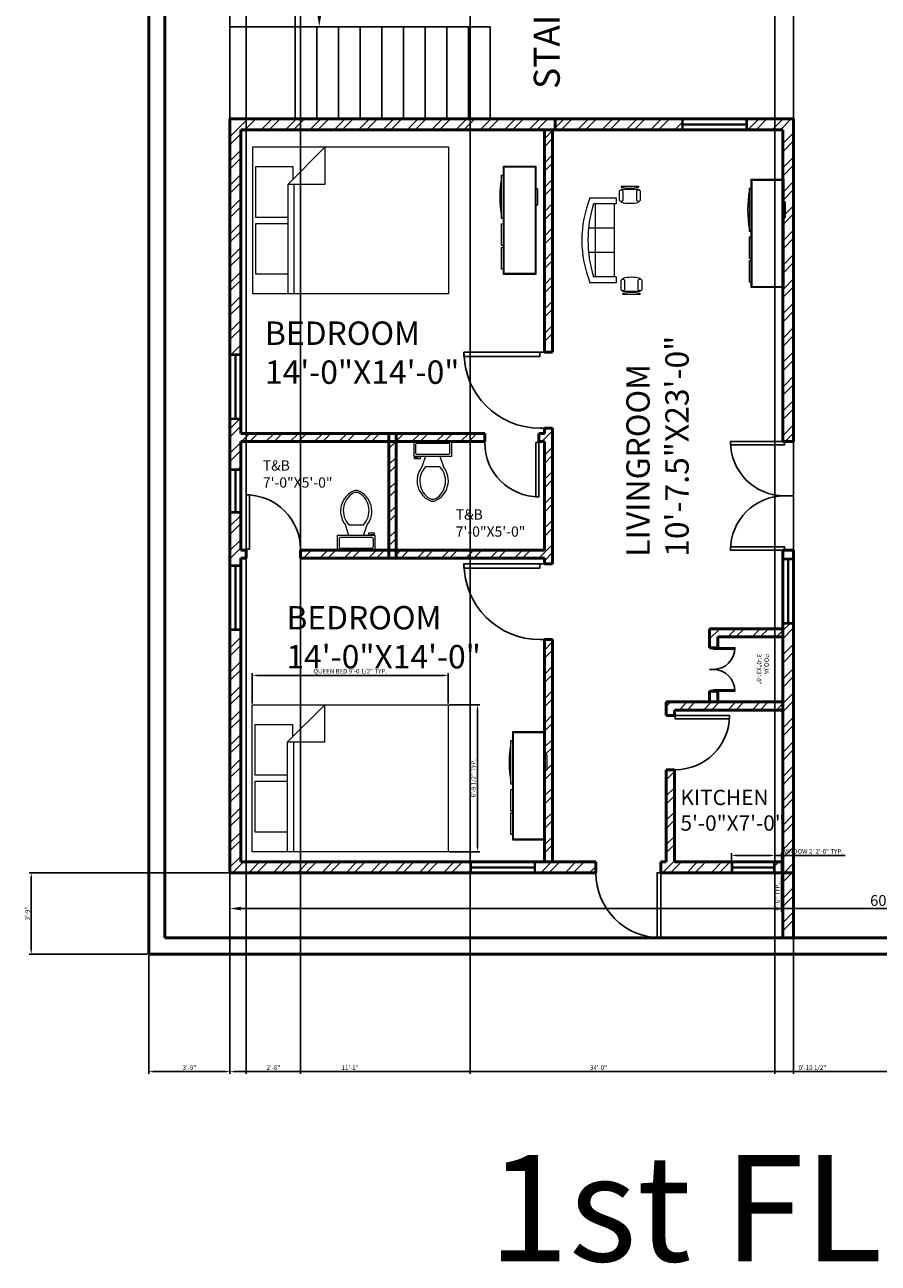
# Model space of a CAD drawing. Units: inches. Extents: x -12550 to 6516, y 1273 to 18700.
# Tile 2 of 19: x 1904 to 2377, y 1273 to 1958. Entities that reach past the tile are written whole.
import ezdxf

# ---------------------------------------------------------------- set-up
doc = ezdxf.new("R2010")
doc.units = ezdxf.units.IN
for name, color, linetype, lineweight in [('A-ANNO-DIMS', 2, 'Continuous', 18), ('A-ANNO-TEXT', 7, 'Continuous', 25), ('A-AREA-IDEN', 1, 'Continuous', 18), ('A-DOOR', 5, 'Continuous', 25), ('A-FLOR-STRS', 6, 'Continuous', 25), ('A-FURN', 8, 'Continuous', 18), ('A-GLAZ', 3, 'Continuous', 25), ('A-WALL', 7, 'Continuous', 50), ('A-WALL-PATT', 8, 'Continuous', 13)]:
    doc.layers.add(name, color=color, linetype=linetype, lineweight=lineweight)
doc.styles.get("Standard").update_dxf_attribs({"font": 'arial.ttf'})
doc.dimstyles.new('ISO-25', dxfattribs={"dimtxt": 2.5, "dimasz": 2.5, "dimexe": 1.25, "dimexo": 0.625, "dimtad": 1, "dimlunit": 4, "dimtxsty": 'Standard', "dimcen": 2.5, "dimadec": 0, "dimazin": 0, "dimtfac": 1, "dimtmove": 0, "dimatfit": 3, "dimfxl": 1, "dimarcsym": 0})

# ---------------------------------------------------------------- blocks, each defined once
blk = doc.blocks.new('*U2')
for p, q in [((0, 0), (0, -5)), ((30, 0), (30, -5))]:
    blk.add_line(p, q)
blk.add_lwpolyline([(0, 0), (0, 30), (1.75, 30), (1.75, 0)], close=True)
blk.add_arc((0, 0), 30, 0, 90)
blk = doc.blocks.new('Bed - Queen')
for p, q in [((0, -80.00003), (0, 0)), ((0, 0), (59.99999, 0)), ((59.99999, 0), (59.99999, -80.00003)), ((7.99999, -1.2), (28.79998, -1.2)), ((7.99999, -14.4), (7.99999, -1.2)), ((28.79998, -1.2), (28.79998, -14.4)), ((31.19999, -1.2), (51.99999, -1.2)), ((31.19999, -14.4), (31.19999, -1.2)), ((51.99999, -1.2), (51.99999, -16.4)), ((0, -14.4), (44.8, -14.4)), ((59.99999, -29.6), (44.8, -14.4)), ((44.8, -14.4), (44.8, -29.6)), ((44.8, -16.8), (0, -16.8)), ((51.99999, -16.4), (46.79936, -16.4)), ((44.8, -29.6), (59.99999, -29.6)), ((59.99999, -80.00003), (0, -80.00003))]:
    blk.add_line(p, q)
blk = doc.blocks.new('Toilet - top')
for p, q in [((9.5, -6), (9.5, -2)), ((-10, -8.5), (-8, -8.5)), ((-10, -9.5), (-10, -8.5)), ((-7, -9.5), (-10, -9.5)), ((-8, -8.5), (-8, -8)), ((-7, -8), (-7, -9.5)), ((-4, -8), (-6, -14)), ((4, -8), (6, -14)), ((4, -14), (-4, -14))]:
    blk.add_line(p, q)
blk.add_lwpolyline([(10.5, -8), (10.5, 0), (-10.5, 0), (-10.5, -8)], close=True)
for points in [[(-9.5, -2), (-9.5, -6)], [(8.5, -1), (-8.5, -1)], [(-8.5, -7), (8.5, -7)]]:
    blk.add_lwpolyline(points)
for centre, radius, start, end in [((-8.62, -1.88), 0.884, 81.8699, 188.1301), ((-8.62, -6.12), 0.884, 171.8699, 278.1301), ((8.62, -1.88), 0.884, 351.8699, 98.1301), ((8.62, -6.12), 0.884, 261.8699, 8.1301), ((3.52, -21.58), 12.17, 141.46911, 247.97143), ((4.2, -21.82), 11.33, 136.36773, 238.94682), ((-3.52, -21.58), 12.17, 292.02843, 38.53071), ((-4.2, -21.82), 11.33, 301.05301, 43.63209), ((0, -27.88), 4, 245.73182, 294.26817), ((0, -29), 4, 254.86053, 285.13947)]:
    blk.add_arc(centre, radius, start, end)
blk = doc.blocks.new('Entertainment Center')
for p, q in [((-4, 0), (-5, -1)), ((4, 0), (-4, 0)), ((5, -1), (4, 0)), ((-17, -19), (-17, -1)), ((-17, -1), (43, -1)), ((-16.5, -18.5), (-16.5, -1.5)), ((-16.5, -1.5), (42.5, -1.5)), ((42.5, -1.5), (42.5, -18.5)), ((43, -1), (43, -19)), ((43, -19), (-17, -19)), ((42.5, -18.5), (-16.5, -18.5)), ((-12, -20), (-12, -19)), ((12, -20), (-12, -20)), ((12, -19), (12, -20)), ((15, -20), (15, -19)), ((27, -20), (15, -20)), ((27, -19), (27, -20)), ((28, -20), (28, -19)), ((40, -20), (28, -20)), ((40, -19), (40, -20))]:
    blk.add_line(p, q)
blk.add_arc((0, 40), 61, 259.6111, 280.3889)
blk = doc.blocks.new('Sofa - Roundback 7 ft.')
for p, q in [((-36.000027, -34), (-36.000027, -11.4696)), ((-12.00002, -32.4421), (-12.00003, -6.5971)), ((11.99997, -32.4421), (11.99998, -6.5971)), ((35.99998, -34), (35.99998, -11.4696)), ((-35.999844, -13.3819), (35.9998, -13.3819)), ((-36.000027, -32.4421), (35.99998, -32.4421))]:
    blk.add_line(p, q)
for points in [[(-36.000027, -34), (-42.000027, -34), (-42.000027, -8)], [(41.99998, -8), (41.99998, -34), (35.99998, -34)]]:
    blk.add_lwpolyline(points)
for centre, radius, start, end in [((0, -114.25), 114.25, 68.43141, 111.5686), ((-0.00001, -127.1968), 121.1968, 72.72033, 107.2797)]:
    blk.add_arc(centre, radius, start, end)
blk = doc.blocks.new('Chair - Desk')
for p, q in [((-8.5, 0), (-8.5, -1)), ((-8.5, 0), (8.5, 0)), ((8.5, 0), (8.5, -1)), ((-10.5, -5), (-10.5, -14)), ((-8.5, -3), (-8.5, -4)), ((-8.5, -3), (8.5, -3)), ((-6.5, -14), (-6.5, -5)), ((-2, -3), (-2, -1.9355)), ((2, -1.9576), (2, -3)), ((6.5, -5), (6.5, -14)), ((8.5, -3), (8.5, -4)), ((10.5, -14), (10.5, -5)), ((-8.5, -15), (-8.5, -16)), ((8.5, -15), (8.5, -16))]:
    blk.add_line(p, q)
for centre, radius, start, end in [((-8.5, -6.5), 2.5, 36.8699, 143.1301), ((0, 34.625), 36.625, 256.5803, 283.4197), ((8.5, -6.5), 2.5, 36.8699, 143.1301), ((-8.5, -12.5), 2.5, 216.8699, 323.1301), ((0, 19.625), 36.625, 256.5803, 283.4197), ((8.5, -12.5), 2.5, 216.8699, 323.1301)]:
    blk.add_arc(centre, radius, start, end)
blk = doc.blocks.new('*D13')
at = {"layer": 'A-ANNO-DIMS', "color": 0, "lineweight": -2, "transparency": 16777216}
for p, q in [((2054.31, 2008.25), (2068.36, 2008.25)), ((2067.11, 2002.25), (2067.11, 1963.25)), ((2054.31, 1957.25), (2068.36, 1957.25))]:
    blk.add_line(p, q, dxfattribs=at)
at = {"layer": 'A-ANNO-DIMS', "color": 0, "transparency": 16777216}
for points in [[(2066.11, 2002.25), (2068.11, 2002.25), (2067.11, 2008.25)], [(2066.11, 1963.25), (2068.11, 1963.25), (2067.11, 1957.25)]]:
    blk.add_solid(points, dxfattribs=at)
at = {"layer": 'Defpoints', "color": 0, "transparency": 16777216}
for p in [(2053.69, 2008.25), (2053.69, 1957.25), (2067.11, 1957.25)]:
    blk.add_point(p, dxfattribs=at)
at = {"layer": 'A-ANNO-DIMS', "color": 0, "transparency": 16777216, "insert": (2063.42, 1982.75), "char_height": 6, "attachment_point": 5, "rotation": 90}
blk.add_mtext('4\'-3"', dxfattribs=at)
blk = doc.blocks.new('*D17')
at = {"layer": 'A-ANNO-DIMS', "color": 0, "lineweight": -2, "transparency": 16777216}
for p, q in [((2017.69, 1488.62), (2017.69, 1468.21)), ((2737.69, 1488.62), (2737.69, 1468.21)), ((2731.69, 1469.46), (2023.69, 1469.46))]:
    blk.add_line(p, q, dxfattribs=at)
at = {"layer": 'A-ANNO-DIMS', "color": 0, "transparency": 16777216}
for points in [[(2023.69, 1470.46), (2023.69, 1468.46), (2017.69, 1469.46)], [(2731.69, 1470.46), (2731.69, 1468.46), (2737.69, 1469.46)]]:
    blk.add_solid(points, dxfattribs=at)
at = {"layer": 'Defpoints', "color": 0, "transparency": 16777216}
for p in [(2017.69, 1489.25), (2737.69, 1489.25), (2017.69, 1469.46)]:
    blk.add_point(p, dxfattribs=at)
at = {"layer": 'A-ANNO-DIMS', "color": 0, "transparency": 16777216, "insert": (2377.69, 1473.15), "char_height": 6, "attachment_point": 5}
blk.add_mtext("60'", dxfattribs=at)
blk = doc.blocks.new('WIN-3FT')
for p, q in [((0, 0), (0, 6)), ((0, 6), (36.02, 6)), ((36.02, 0), (0, 0)), ((0.5, 0), (0.5, 6)), ((35.52, 3.2), (0.5, 3.2)), ((35.52, 2.8), (0.5, 2.8)), ((35.52, 6), (35.52, 0)), ((36.02, 6), (36.02, 0))]:
    blk.add_line(p, q)
blk = doc.blocks.new('WIN-2FT')
for p, q in [((0, 0), (0, 24.02)), ((0, 24.02), (6, 24.02)), ((0, 23.52), (6, 23.52)), ((2.8, 0.5), (2.8, 23.52)), ((3.2, 0.5), (3.2, 23.52)), ((6, 24.02), (6, 0)), ((6, 0.5), (0, 0.5)), ((6, 0), (0, 0))]:
    blk.add_line(p, q)
blk = doc.blocks.new('*D65')
at = {"layer": 'A-ANNO-DIMS', "color": 0, "lineweight": -2, "transparency": 16777216}
for p, q in [((2295.28, 1495.87), (2295.28, 1500.1)), ((2297.78, 1498.85), (2316.79, 1498.85)), ((2319.29, 1495.87), (2319.29, 1500.1)), ((2319.29, 1498.85), (2358.26, 1498.85))]:
    blk.add_line(p, q, dxfattribs=at)
at = {"layer": 'A-ANNO-DIMS', "color": 0, "transparency": 16777216}
for points in [[(2297.78, 1499.27), (2297.78, 1498.43), (2295.28, 1498.85)], [(2316.79, 1499.27), (2316.79, 1498.43), (2319.29, 1498.85)]]:
    blk.add_solid(points, dxfattribs=at)
at = {"layer": 'Defpoints', "color": 0, "transparency": 16777216}
for p in [(2295.28, 1495.25), (2319.29, 1498.85), (2319.29, 1495.25)]:
    blk.add_point(p, dxfattribs=at)
at = {"layer": 'A-ANNO-DIMS', "color": 0, "transparency": 16777216, "insert": (2340.03, 1500.77), "char_height": 2.5, "attachment_point": 5}
blk.add_mtext('WINDOW 2\' 2\'-0" TYP.', dxfattribs=at)
blk = doc.blocks.new('*D66')
at = {"layer": 'A-ANNO-DIMS', "color": 0, "lineweight": -2, "transparency": 16777216}
for p, q in [((2319.92, 1495.25), (2324.15, 1495.25)), ((2322.9, 1497.75), (2322.9, 1500.25)), ((2322.9, 1495.25), (2322.9, 1489.25)), ((2319.92, 1489.25), (2324.15, 1489.25)), ((2322.9, 1486.75), (2322.9, 1467.76))]:
    blk.add_line(p, q, dxfattribs=at)
at = {"layer": 'A-ANNO-DIMS', "color": 0, "transparency": 16777216}
for points in [[(2322.48, 1497.75), (2323.31, 1497.75), (2322.9, 1495.25)], [(2322.48, 1486.75), (2323.31, 1486.75), (2322.9, 1489.25)]]:
    blk.add_solid(points, dxfattribs=at)
at = {"layer": 'Defpoints', "color": 0, "transparency": 16777216}
for p in [(2319.29, 1495.25), (2319.29, 1489.25), (2322.9, 1489.25)]:
    blk.add_point(p, dxfattribs=at)
at = {"layer": 'A-ANNO-DIMS', "color": 0, "transparency": 16777216, "insert": (2321, 1476), "char_height": 2.5, "attachment_point": 5, "rotation": 90}
blk.add_mtext('0\'-6" TYP.', dxfattribs=at)
blk = doc.blocks.new('*D69')
at = {"layer": 'A-ANNO-DIMS', "color": 0, "lineweight": -2, "transparency": 16777216}
for p, q in [((2030.04, 1582.83), (2030.04, 1599.71)), ((2135.92, 1598.46), (2032.54, 1598.46)), ((2138.42, 1582.83), (2138.42, 1599.71))]:
    blk.add_line(p, q, dxfattribs=at)
at = {"layer": 'A-ANNO-DIMS', "color": 0, "transparency": 16777216}
for points in [[(2032.54, 1598.88), (2032.54, 1598.05), (2030.04, 1598.46)], [(2135.92, 1598.88), (2135.92, 1598.05), (2138.42, 1598.46)]]:
    blk.add_solid(points, dxfattribs=at)
at = {"layer": 'Defpoints', "color": 0, "transparency": 16777216}
for p in [(2030.04, 1598.46), (2030.04, 1582.2), (2138.42, 1582.2)]:
    blk.add_point(p, dxfattribs=at)
at = {"layer": 'A-ANNO-DIMS', "color": 0, "transparency": 16777216, "insert": (2084.23, 1600.46), "char_height": 2.5, "attachment_point": 5}
blk.add_mtext('QUEEN BED 9\'-0 1/2" TYP.', dxfattribs=at)
blk = doc.blocks.new('*D70')
at = {"layer": 'A-ANNO-DIMS', "color": 0, "lineweight": -2, "transparency": 16777216}
for p, q in [((2139.05, 1582.2), (2155.93, 1582.2)), ((2154.68, 1503.41), (2154.68, 1579.7)), ((2139.05, 1500.91), (2155.93, 1500.91))]:
    blk.add_line(p, q, dxfattribs=at)
at = {"layer": 'A-ANNO-DIMS', "color": 0, "transparency": 16777216}
for points in [[(2154.27, 1579.7), (2155.1, 1579.7), (2154.68, 1582.2)], [(2154.27, 1503.41), (2155.1, 1503.41), (2154.68, 1500.91)]]:
    blk.add_solid(points, dxfattribs=at)
at = {"layer": 'Defpoints', "color": 0, "transparency": 16777216}
for p in [(2138.42, 1582.2), (2154.68, 1582.2), (2138.42, 1500.91)]:
    blk.add_point(p, dxfattribs=at)
at = {"layer": 'A-ANNO-DIMS', "color": 0, "transparency": 16777216, "insert": (2152.76, 1541.56), "char_height": 2.5, "attachment_point": 5, "rotation": 90}
blk.add_mtext('6\'-9 1/2" TYP.', dxfattribs=at)
blk = doc.blocks.new('*D96')
at = {"layer": 'A-ANNO-DIMS', "color": 0, "lineweight": -2, "transparency": 16777216}
for p, q in [((2017.69, 1488.62), (2017.69, 1378)), ((1972.69, 1443.62), (1972.69, 1378)), ((1975.19, 1379.25), (2015.19, 1379.25))]:
    blk.add_line(p, q, dxfattribs=at)
at = {"layer": 'A-ANNO-DIMS', "color": 0, "transparency": 16777216}
for points in [[(1975.19, 1379.66), (1975.19, 1378.83), (1972.69, 1379.25)], [(2015.19, 1379.66), (2015.19, 1378.83), (2017.69, 1379.25)]]:
    blk.add_solid(points, dxfattribs=at)
at = {"layer": 'Defpoints', "color": 0, "transparency": 16777216}
for p in [(2017.69, 1489.25), (1972.69, 1444.25), (2017.69, 1379.25)]:
    blk.add_point(p, dxfattribs=at)
at = {"layer": 'A-ANNO-DIMS', "color": 0, "transparency": 16777216, "insert": (1995.19, 1381.15), "char_height": 2.5, "attachment_point": 5}
blk.add_mtext('3\'-9"', dxfattribs=at)
blk = doc.blocks.new('*D97')
at = {"layer": 'A-ANNO-DIMS', "color": 0, "lineweight": -2, "transparency": 16777216}
for p, q in [((2017.69, 1488.62), (2017.69, 1378)), ((2425.69, 1488.62), (2425.69, 1378)), ((2020.19, 1379.25), (2423.19, 1379.25))]:
    blk.add_line(p, q, dxfattribs=at)
at = {"layer": 'A-ANNO-DIMS', "color": 0, "transparency": 16777216}
for points in [[(2020.19, 1379.66), (2020.19, 1378.83), (2017.69, 1379.25)], [(2423.19, 1379.66), (2423.19, 1378.83), (2425.69, 1379.25)]]:
    blk.add_solid(points, dxfattribs=at)
at = {"layer": 'Defpoints', "color": 0, "transparency": 16777216}
for p in [(2017.69, 1489.25), (2425.69, 1489.25), (2425.69, 1379.25)]:
    blk.add_point(p, dxfattribs=at)
at = {"layer": 'A-ANNO-DIMS', "color": 0, "transparency": 16777216, "insert": (2221.69, 1381.15), "char_height": 2.5, "attachment_point": 5}
blk.add_mtext('34\'-0"', dxfattribs=at)
blk = doc.blocks.new('*D101')
at = {"layer": 'A-ANNO-DIMS', "color": 0, "lineweight": -2, "transparency": 16777216}
for p, q in [((2017.06, 1489.25), (1906.44, 1489.25)), ((1907.69, 1446.75), (1907.69, 1486.75)), ((1972.06, 1444.25), (1906.44, 1444.25))]:
    blk.add_line(p, q, dxfattribs=at)
at = {"layer": 'A-ANNO-DIMS', "color": 0, "transparency": 16777216}
for points in [[(1907.27, 1486.75), (1908.11, 1486.75), (1907.69, 1489.25)], [(1907.27, 1446.75), (1908.11, 1446.75), (1907.69, 1444.25)]]:
    blk.add_solid(points, dxfattribs=at)
at = {"layer": 'Defpoints', "color": 0, "transparency": 16777216}
for p in [(1907.69, 1489.25), (2017.69, 1489.25), (1972.69, 1444.25)]:
    blk.add_point(p, dxfattribs=at)
at = {"layer": 'A-ANNO-DIMS', "color": 0, "transparency": 16777216, "insert": (1905.79, 1466.75), "char_height": 2.5, "attachment_point": 5, "rotation": 90}
blk.add_mtext('3\'-9"', dxfattribs=at)
blk = doc.blocks.new('*D136')
at = {"layer": 'A-ANNO-DIMS', "color": 0, "lineweight": -2, "transparency": 16777216}
for p, q in [((2017.69, 2055.62), (2017.69, 1378)), ((2150.64, 2055.62), (2150.64, 1378)), ((2020.19, 1379.25), (2148.14, 1379.25))]:
    blk.add_line(p, q, dxfattribs=at)
at = {"layer": 'A-ANNO-DIMS', "color": 0, "transparency": 16777216}
for points in [[(2020.19, 1379.66), (2020.19, 1378.83), (2017.69, 1379.25)], [(2148.14, 1379.66), (2148.14, 1378.83), (2150.64, 1379.25)]]:
    blk.add_solid(points, dxfattribs=at)
at = {"layer": 'Defpoints', "color": 0, "transparency": 16777216}
for p in [(2017.69, 2056.25), (2150.64, 2056.25), (2150.64, 1379.25)]:
    blk.add_point(p, dxfattribs=at)
at = {"layer": 'A-ANNO-DIMS', "color": 0, "transparency": 16777216, "insert": (2084.16, 1381.13), "char_height": 2.5, "attachment_point": 5}
blk.add_mtext('11\'-1"', dxfattribs=at)
blk = doc.blocks.new('*D137')
at = {"layer": 'A-ANNO-DIMS', "color": 0, "lineweight": -2, "transparency": 16777216}
for p, q in [((2319.29, 2055.62), (2319.29, 1378)), ((2329.69, 2055.62), (2329.69, 1378)), ((2321.79, 1379.25), (2327.19, 1379.25)), ((2329.69, 1379.25), (2347.85, 1379.25))]:
    blk.add_line(p, q, dxfattribs=at)
at = {"layer": 'A-ANNO-DIMS', "color": 0, "transparency": 16777216}
for points in [[(2321.79, 1379.66), (2321.79, 1378.83), (2319.29, 1379.25)], [(2327.19, 1379.66), (2327.19, 1378.83), (2329.69, 1379.25)]]:
    blk.add_solid(points, dxfattribs=at)
at = {"layer": 'Defpoints', "color": 0, "transparency": 16777216}
for p in [(2319.29, 2056.25), (2329.69, 2056.25), (2329.69, 1379.25)]:
    blk.add_point(p, dxfattribs=at)
at = {"layer": 'A-ANNO-DIMS', "color": 0, "transparency": 16777216, "insert": (2340.02, 1381.16), "char_height": 2.5, "attachment_point": 5}
blk.add_mtext('0\'-10 1/2"', dxfattribs=at)
blk = doc.blocks.new('*D142')
at = {"layer": 'A-ANNO-DIMS', "color": 0, "lineweight": -2, "transparency": 16777216}
for p, q in [((2026.69, 2234.12), (2026.69, 1378)), ((2056.69, 2234.12), (2056.69, 1378)), ((2029.19, 1379.25), (2054.19, 1379.25))]:
    blk.add_line(p, q, dxfattribs=at)
at = {"layer": 'A-ANNO-DIMS', "color": 0, "transparency": 16777216}
for points in [[(2029.19, 1379.66), (2029.19, 1378.83), (2026.69, 1379.25)], [(2054.19, 1379.66), (2054.19, 1378.83), (2056.69, 1379.25)]]:
    blk.add_solid(points, dxfattribs=at)
at = {"layer": 'Defpoints', "color": 0, "transparency": 16777216}
for p in [(2026.69, 2234.75), (2056.69, 2234.75), (2056.69, 1379.25)]:
    blk.add_point(p, dxfattribs=at)
at = {"layer": 'A-ANNO-DIMS', "color": 0, "transparency": 16777216, "insert": (2041.69, 1381.15), "char_height": 2.5, "attachment_point": 5}
blk.add_mtext('2\'-6"', dxfattribs=at)

msp = doc.modelspace()

# ---------------------------------------------------------------- hatches: boundary and pattern name
at = {"layer": 'A-WALL-PATT'}
h = msp.add_hatch(dxfattribs=at)
h.set_pattern_fill('ANSI32', color=256)
h.paths.add_polyline_path([(2023.689, 1900.247), (2197.689, 1900.247), (2197.689, 1906.247), (2017.689, 1906.247), (2017.689, 1776.138), (2023.689, 1776.138)])
h = msp.add_hatch(dxfattribs=at)
h.set_pattern_fill('ANSI32', color=256)
h.paths.add_polyline_path([(2267.94, 1906.247), (2197.689, 1906.247), (2197.689, 1900.247), (2267.94, 1900.247)])
h = msp.add_hatch(dxfattribs=at)
h.set_pattern_fill('ANSI32', color=256)
h.paths.add_polyline_path([(2329.689, 1906.247), (2303.958, 1906.247), (2303.958, 1900.247), (2323.689, 1900.247), (2323.689, 1872.972), (2324.189, 1872.972), (2324.189, 1860.972), (2325.189, 1859.972), (2325.189, 1851.972), (2324.189, 1850.972), (2324.189, 1812.972), (2323.689, 1727.747), (2324.689, 1727.747), (2329.689, 1727.747)])
h = msp.add_hatch(dxfattribs=at)
h.set_pattern_fill('ANSI32', color=256)
h.paths.add_polyline_path([(2196.189, 1900.247), (2191.689, 1900.247), (2191.689, 1777.247), (2196.189, 1777.247)], flags=17)
h = msp.add_hatch(dxfattribs=at)
h.set_pattern_fill('ANSI32', color=256)
h.paths.add_polyline_path([(2105.689, 1732.247), (2023.689, 1732.247), (2023.689, 1740.121), (2017.689, 1740.121), (2017.689, 1712.466), (2023.689, 1712.466), (2023.689, 1727.747), (2105.689, 1727.747)])
h = msp.add_hatch(dxfattribs=at)
h.set_pattern_fill('ANSI32', color=256)
h.paths.add_polyline_path([(2196.189, 1735.247), (2191.689, 1735.247), (2191.689, 1732.247), (2188.689, 1732.247), (2188.689, 1727.747), (2191.689, 1727.747), (2191.689, 1667.747), (2109.689, 1667.747), (2109.689, 1663.247), (2191.689, 1663.247), (2191.689, 1660.247), (2196.189, 1660.247)])
h = msp.add_hatch(dxfattribs=at)
h.set_pattern_fill('ANSI32', color=256)
h.paths.add_polyline_path([(2109.689, 1727.747), (2105.689, 1727.747), (2105.689, 1667.747), (2109.689, 1667.747)])
h = msp.add_hatch(dxfattribs=at)
h.set_pattern_fill('ANSI32', color=256)
h.paths.add_polyline_path([(2158.689, 1732.247), (2109.689, 1732.247), (2109.689, 1727.747), (2158.689, 1727.747)], flags=17)
h = msp.add_hatch(dxfattribs=at)
h.set_pattern_fill('ANSI32', color=256)
h.paths.add_polyline_path([(2023.689, 1688.449), (2017.689, 1688.449), (2017.689, 1659.453), (2023.689, 1659.453), (2023.689, 1663.247), (2026.689, 1663.247), (2026.689, 1667.747), (2023.689, 1667.747)])
h = msp.add_hatch(dxfattribs=at)
h.set_pattern_fill('ANSI32', color=256)
h.paths.add_polyline_path([(2105.689, 1667.747), (2056.689, 1667.747), (2056.689, 1663.247), (2105.689, 1663.247)])
h = msp.add_hatch(dxfattribs=at)
h.set_pattern_fill('ANSI32', color=256)
h.paths.add_polyline_path([(2323.689, 1624.247), (2283.189, 1624.247), (2283.189, 1613.747), (2285.189, 1613.747), (2287.689, 1613.747), (2287.689, 1619.747), (2323.689, 1619.747)])
h = msp.add_hatch(dxfattribs=at)
h.set_pattern_fill('ANSI32', color=256)
h.paths.add_polyline_path([(2329.689, 1627.032), (2323.689, 1627.032), (2323.689, 1495.247), (2319.294, 1495.247), (2319.294, 1489.247), (2329.689, 1489.247)])
h = msp.add_hatch(dxfattribs=at)
h.set_pattern_fill('ANSI32', color=256)
h.paths.add_polyline_path([(2023.689, 1623.435), (2017.689, 1623.435), (2017.689, 1489.247), (2150.64, 1489.247), (2150.64, 1495.247), (2023.689, 1495.247)])
h = msp.add_hatch(dxfattribs=at)
h.set_pattern_fill('ANSI32', color=256)
h.paths.add_polyline_path([(2196.189, 1618.247), (2191.689, 1618.247), (2191.689, 1567.365), (2192.189, 1567.365), (2192.189, 1555.365), (2193.189, 1554.365), (2193.189, 1546.365), (2192.189, 1545.365), (2192.189, 1507.365), (2191.689, 1495.247), (2196.189, 1495.247)])
h = msp.add_hatch(dxfattribs=at)
h.set_pattern_fill('ANSI32', color=256)
h.paths.add_polyline_path([(2323.689, 1583.747), (2259.189, 1583.747), (2259.189, 1576.247), (2263.689, 1576.247), (2263.689, 1579.247), (2323.689, 1579.247)])
h = msp.add_hatch(dxfattribs=at)
h.set_pattern_fill('ANSI32', color=256)
h.paths.add_polyline_path([(2295.277, 1495.247), (2263.689, 1495.247), (2263.689, 1546.247), (2259.189, 1546.247), (2259.189, 1495.247), (2256.189, 1495.247), (2256.189, 1489.247), (2295.277, 1489.247)])
h = msp.add_hatch(dxfattribs=at)
h.set_pattern_fill('ANSI32', color=256)
h.paths.add_polyline_path([(2220.189, 1495.247), (2186.657, 1495.247), (2186.657, 1489.247), (2220.189, 1489.247)])
h = msp.add_hatch(dxfattribs=at)
h.set_pattern_fill('ANSI32', color=256)
h.paths.add_polyline_path([(2329.689, 1489.247), (2323.689, 1489.247), (2323.689, 1453.247), (2329.689, 1453.247)])

# ---------------------------------------------------------------- linework, layer by layer
at = {"layer": 'A-FLOR-STRS'}
for p, q in [((2017.689, 2056.247), (2017.689, 1906.247)), ((2053.689, 2056.247), (2053.689, 1906.247)), ((2017.689, 1957.247), (2161.689, 1957.247)), ((2065.689, 1957.247), (2065.689, 1906.247)), ((2077.689, 1957.247), (2077.689, 1906.247)), ((2089.689, 1957.247), (2089.689, 1906.247)), ((2101.689, 1957.247), (2101.689, 1906.247)), ((2113.689, 1957.247), (2113.689, 1906.247)), ((2125.689, 1957.247), (2125.689, 1906.247)), ((2137.689, 1957.247), (2137.689, 1906.247)), ((2149.689, 1957.247), (2149.689, 1906.247)), ((2161.689, 1957.247), (2161.689, 1906.247)), ((2017.689, 1906.247), (2197.689, 1906.247))]:
    msp.add_line(p, q, dxfattribs=at)
at = {"layer": 'A-WALL'}
for p, q in [((1972.689, 1444.247), (1972.689, 2518.247)), ((1981.689, 1453.247), (1981.689, 2509.247)), ((2017.689, 1489.247), (2017.689, 1906.247)), ((2329.689, 1906.247), (2017.689, 1906.247)), ((2197.689, 1900.247), (2197.689, 1906.247)), ((2329.689, 1727.747), (2329.689, 1906.247)), ((2023.689, 1732.247), (2023.689, 1900.247)), ((2323.689, 1900.247), (2023.689, 1900.247)), ((2191.689, 1777.247), (2191.689, 1900.247)), ((2196.189, 1777.247), (2196.189, 1900.247)), ((2323.689, 1727.747), (2323.689, 1900.247)), ((2196.189, 1777.247), (2191.689, 1777.247)), ((2191.689, 1732.247), (2191.689, 1735.247)), ((2191.689, 1735.247), (2196.189, 1735.247)), ((2191.689, 1732.247), (2191.689, 1735.247)), ((2196.189, 1660.247), (2196.189, 1735.247)), ((2158.689, 1732.247), (2023.689, 1732.247)), ((2158.689, 1727.747), (2023.689, 1727.747)), ((2023.689, 1667.747), (2023.689, 1727.747)), ((2105.689, 1663.247), (2105.689, 1732.247)), ((2109.689, 1663.247), (2109.689, 1732.247)), ((2158.689, 1727.747), (2158.689, 1732.247)), ((2191.689, 1732.247), (2188.689, 1732.247)), ((2191.689, 1732.247), (2188.689, 1732.247)), ((2188.689, 1732.247), (2188.689, 1727.747)), ((2191.689, 1727.747), (2188.689, 1727.747)), ((2191.689, 1667.747), (2191.689, 1727.747)), ((2329.689, 1727.747), (2323.689, 1727.747)), ((2026.689, 1667.747), (2023.689, 1667.747)), ((2026.689, 1663.247), (2026.689, 1667.747)), ((2191.689, 1667.747), (2056.689, 1667.747)), ((2056.689, 1667.747), (2191.689, 1667.747)), ((2056.689, 1667.747), (2056.689, 1663.247)), ((2323.689, 1453.247), (2323.689, 1667.747)), ((2329.689, 1667.747), (2323.689, 1667.747)), ((2329.689, 1489.247), (2329.689, 1667.747)), ((2023.689, 1495.247), (2023.689, 1663.247)), ((2023.689, 1663.247), (2026.689, 1663.247)), ((2026.689, 1663.247), (2023.689, 1663.247)), ((2191.689, 1663.247), (2056.689, 1663.247)), ((2191.689, 1660.247), (2191.689, 1663.247)), ((2196.189, 1660.247), (2191.689, 1660.247)), ((2196.189, 1663.247), (2196.189, 1660.247)), ((2323.689, 1624.247), (2283.189, 1624.247)), ((2283.189, 1613.747), (2283.189, 1624.247)), ((2191.689, 1495.247), (2191.689, 1618.247)), ((2191.689, 1618.247), (2196.189, 1618.247)), ((2196.189, 1495.247), (2196.189, 1618.247)), ((2323.689, 1619.747), (2287.689, 1619.747)), ((2287.689, 1613.747), (2287.689, 1619.747)), ((2283.189, 1613.747), (2287.689, 1613.747)), ((2283.189, 1583.747), (2283.189, 1589.747)), ((2287.689, 1589.747), (2283.189, 1589.747)), ((2287.689, 1583.747), (2287.689, 1589.747)), ((2287.689, 1583.747), (2287.689, 1589.747)), ((2323.689, 1583.747), (2259.189, 1583.747)), ((2259.189, 1576.247), (2259.189, 1583.747)), ((2283.189, 1583.747), (2283.189, 1588.747)), ((2263.689, 1576.247), (2259.189, 1576.247)), ((2323.689, 1579.247), (2263.689, 1579.247)), ((2263.689, 1579.247), (2263.689, 1576.247)), ((2263.689, 1576.247), (2263.689, 1579.247)), ((2259.189, 1495.247), (2259.189, 1546.247)), ((2259.189, 1546.247), (2263.689, 1546.247)), ((2263.689, 1495.247), (2263.689, 1546.247)), ((2220.189, 1495.247), (2023.689, 1495.247)), ((2220.189, 1495.247), (2196.189, 1495.247)), ((2220.189, 1489.247), (2220.189, 1495.247)), ((2259.189, 1495.247), (2256.189, 1495.247)), ((2259.189, 1495.247), (2256.189, 1495.247)), ((2256.189, 1495.247), (2256.189, 1489.247)), ((2323.689, 1495.247), (2263.689, 1495.247)), ((2220.189, 1489.247), (2017.689, 1489.247)), ((2329.689, 1489.247), (2256.189, 1489.247)), ((2329.689, 1489.247), (2329.689, 1453.247)), ((1981.689, 1453.247), (2773.689, 1453.247)), ((2520.189, 1453.247), (2256.189, 1453.247)), ((1972.689, 1444.247), (2782.689, 1444.247))]:
    msp.add_line(p, q, dxfattribs=at)

# ---------------------------------------------------------------- block references
at = {"layer": 'A-DOOR'}
for p, xscale, yscale, zscale, rotation in [((2189.189, 1777.247), -1.4, 1.4, 1.4, 90), ((2189.189, 1660.247), -1.4, 1.4, 1.4, 90), ((2285.189, 1613.747), 0.399999999999997, 0.399999999999997, 0.399999999999997, 270), ((2285.189, 1589.747), -0.399999999999997, 0.399999999999997, 0.399999999999997, 270), ((2256.189, 1489.247), 1.199999999999999, 1.199999999999999, 1.199999999999999, 180)]:
    msp.add_blockref('*U2', p, dxfattribs=dict(at, xscale=xscale, yscale=yscale, zscale=zscale, rotation=rotation))
for p, rotation in [((2188.689, 1727.247), 180), ((2324.689, 1667.747), 90), ((2264.189, 1576.247), 270)]:
    msp.add_blockref('*U2', p, dxfattribs=dict(at, rotation=rotation))
at = {"layer": 'A-DOOR', "xscale": -1, "rotation": 90}
msp.add_blockref('*U2', (2324.689, 1727.747), dxfattribs=at)
at = {"layer": 'A-DOOR'}
msp.add_blockref('*U2', (2026.689, 1668.247), dxfattribs=at)
at = {"layer": 'A-FURN'}
for name, p, xscale, yscale, zscale, rotation in [('Bed - Queen', (2030.339, 1809.493), 1.354827908062564, 1.354827908062564, 1.354827908062564, 90), ('Sofa - Roundback 7 ft.', (2212.448, 1839.138), 0.5595223685495907, 0.5595223685495907, 0.5595223685495907, 90), ('Chair - Desk', (2239.887, 1809.138), 0.5595223685495907, 0.5595223685495907, 0.5595223685495907, 180), ('Bed - Queen', (2030.038, 1500.915), 1.354827908062564, 1.354827908062564, 1.354827908062564, 90)]:
    msp.add_blockref(name, p, dxfattribs=dict(at, xscale=xscale, yscale=yscale, zscale=zscale, rotation=rotation))
for name, p, rotation in [('Entertainment Center', (2188.03, 1863.204), 270), ('Entertainment Center', (2325.189, 1855.972), 270), ('Toilet - top', (2087.536, 1667.747), 180), ('Entertainment Center', (2193.189, 1550.365), 270)]:
    msp.add_blockref(name, p, dxfattribs=dict(at, rotation=rotation))
at = {"layer": 'A-FURN', "xscale": 0.5595223685495907, "yscale": 0.5595223685495907, "zscale": 0.5595223685495907}
msp.add_blockref('Chair - Desk', (2239.033, 1869.122), dxfattribs=at)
at = {"layer": 'A-FURN'}
msp.add_blockref('Toilet - top', (2129.9, 1727.747), dxfattribs=at)
at = {"layer": 'A-GLAZ'}
for name, p, rotation in [('WIN-3FT', (2303.957, 1906.247), 180), ('WIN-3FT', (2023.689, 1740.121), 89.99999999999895), ('WIN-2FT', (2023.689, 1712.467), 180), ('WIN-3FT', (2023.689, 1623.436), 90.00000000000024), ('WIN-3FT', (2329.689, 1627.032), 90.000000000002), ('WIN-3FT', (2186.657, 1495.247), 180), ('WIN-2FT', (2295.276, 1495.247), 269.9999999999929)]:
    msp.add_blockref(name, p, dxfattribs=dict(at, rotation=rotation))

# ---------------------------------------------------------------- texts
at = {"layer": 'A-ANNO-TEXT', "insert": (2160.68, 1333.138), "char_height": 58.816, "attachment_point": 1}
msp.add_mtext('1st FLOOR', dxfattribs=at)
at = {"layer": 'A-AREA-IDEN', "attachment_point": 1}
for s, width, gutter_width, insert, char_height, rotation in [('STAIRCASE', 2.19144, 71.795, (2185.866, 1922.837), 14.3589, 90), ('POOJA\\P3\'-0"X3\'-0"', 0.78585, 12.5, (2316.065, 1610.304), 2.5, 269.183853)]:
    msp.add_mtext_dynamic_manual_height_columns(s, width=width, gutter_width=gutter_width, heights=[0], dxfattribs=dict(at, insert=insert, char_height=char_height, rotation=rotation))
at = {"layer": 'A-AREA-IDEN', "char_height": 12.93169, "attachment_point": 1}
for insert in [(2037.025, 1794.217), (2048.907, 1636.812)]:
    msp.add_mtext('BEDROOM\\P14\'-0"X14\'-0"', dxfattribs=dict(at, insert=insert))
at = {"layer": 'A-AREA-IDEN', "insert": (2237.095, 1664.034), "char_height": 12.93169, "attachment_point": 1, "rotation": 90}
msp.add_mtext('LIVINGROOM\\P10\'-7.5"X23\'-0"', dxfattribs=at)
at = {"layer": 'A-AREA-IDEN', "attachment_point": 1}
for s, width, gutter_width, insert, char_height in [('T&B\\P7\'-0"X5\'-0"', 4.19569, 28.328, (2035.864, 1717.416), 5.66556), ('T&B\\P7\'-0"X5\'-0"', 4.19569, 28.328, (2142.626, 1690.282), 5.66556), ('KITCHEN\\P5\'-0"X7\'-0"', 1.29487, 42.422, (2267.01, 1535.176), 8.48435)]:
    msp.add_mtext_dynamic_manual_height_columns(s, width=width, gutter_width=gutter_width, heights=[0], dxfattribs=dict(at, insert=insert, char_height=char_height))

# ---------------------------------------------------------------- dimensions: what is measured, and where the dimension line sits
at = {"layer": 'A-ANNO-DIMS'}
for base, p1, p2, override, picture, middle in [((2056.689, 1379.247), (2026.689, 2234.747), (2056.689, 2234.747), {"dimdec": 1, "dimlfac": 1, "dimrnd": 0, "dimzin": 1, "dimdsep": 46, "dimlunit": 4, "dimfrac": 2}, '*D142', (2041.689, 1381.149)), ((2150.64, 1379.247), (2017.689, 2056.247), (2150.64, 2056.247), {"dimdec": 1, "dimlfac": 1, "dimrnd": 0, "dimzin": 1, "dimdsep": 46, "dimlunit": 4, "dimfrac": 2}, '*D136', (2084.164, 1381.127)), ((2329.689, 1379.247), (2319.294, 2056.247), (2329.689, 2056.247), {"dimdec": 1, "dimlfac": 1, "dimrnd": 0, "dimzin": 1, "dimdsep": 46, "dimlunit": 4, "dimfrac": 2}, '*D137', (2340.02, 1381.165)), ((2017.689, 1379.247), (1972.689, 1444.247), (2017.689, 1489.247), {"dimdec": 1, "dimlfac": 1, "dimrnd": 0, "dimzin": 1, "dimdsep": 46, "dimlunit": 4, "dimfrac": 2}, '*D96', (1995.189, 1381.15)), ((2017.689, 1469.461), (2737.689, 1489.247), (2017.689, 1489.247), {"dimtxt": 6, "dimasz": 6, "dimclrd": 0, "dimclre": 0, "dimclrt": 0}, '*D17', (2377.689, 1473.15)), ((2425.689, 1379.247), (2017.689, 1489.247), (2425.689, 1489.247), {"dimdec": 1, "dimlfac": 1, "dimrnd": 0, "dimzin": 1, "dimdsep": 46, "dimlunit": 4, "dimfrac": 2}, '*D97', (2221.689, 1381.15))]:
    dim = msp.add_linear_dim(base=base, p1=p1, p2=p2, dimstyle='ISO-25', override=override, dxfattribs=at)
    dim.commit()
    dim.dimension.update_dxf_attribs({"geometry": picture, "text_midpoint": middle})
for base, p1, p2, override, picture, middle in [((2067.111, 1957.247), (2053.689, 2008.247), (2053.689, 1957.247), {"dimtxt": 6, "dimasz": 6, "dimclrd": 0, "dimclre": 0, "dimclrt": 0}, '*D13', (2063.42, 1982.747)), ((1907.689, 1489.247), (1972.689, 1444.247), (2017.689, 1489.247), {"dimdec": 1, "dimlfac": 1, "dimrnd": 0, "dimzin": 1, "dimdsep": 46, "dimlunit": 4, "dimfrac": 2}, '*D101', (1905.787, 1466.747))]:
    dim = msp.add_linear_dim(base=base, p1=p1, p2=p2, angle=90, dimstyle='ISO-25', override=override, dxfattribs=at)
    dim.commit()
    dim.dimension.update_dxf_attribs({"geometry": picture, "text_midpoint": middle})
for base, p1, p2, angle, text, picture, middle in [((2030.038, 1598.462), (2138.424, 1582.204), (2030.038, 1582.204), 180, 'QUEEN BED <> TYP.', '*D69', (2084.231, 1600.457)), ((2154.682, 1582.204), (2138.424, 1500.915), (2138.424, 1582.204), 90, '<> TYP.', '*D70', (2152.764, 1541.559)), ((2322.897, 1489.247), (2319.294, 1495.247), (2319.294, 1489.247), 270, '<> TYP.', '*D66', (2320.995, 1476.003))]:
    dim = msp.add_linear_dim(base=base, p1=p1, p2=p2, angle=angle, text=text, dimstyle='ISO-25', override={"dimdec": 1, "dimrnd": 0, "dimzin": 1, "dimlunit": 4, "dimfrac": 2}, dxfattribs=at)
    dim.commit()
    dim.dimension.update_dxf_attribs({"geometry": picture, "text_midpoint": middle})
dim = msp.add_linear_dim(base=(2319.294, 1498.85), p1=(2295.277, 1495.247), p2=(2319.294, 1495.247), text="WINDOW 2' <> TYP.", dimstyle='ISO-25', override={"dimdec": 1, "dimrnd": 0, "dimzin": 1, "dimlunit": 4, "dimfrac": 2}, dxfattribs=at)
dim.commit()
dim.dimension.update_dxf_attribs({"geometry": '*D65', "text_midpoint": (2340.026, 1500.768)})

doc.saveas('drawing.dxf')
